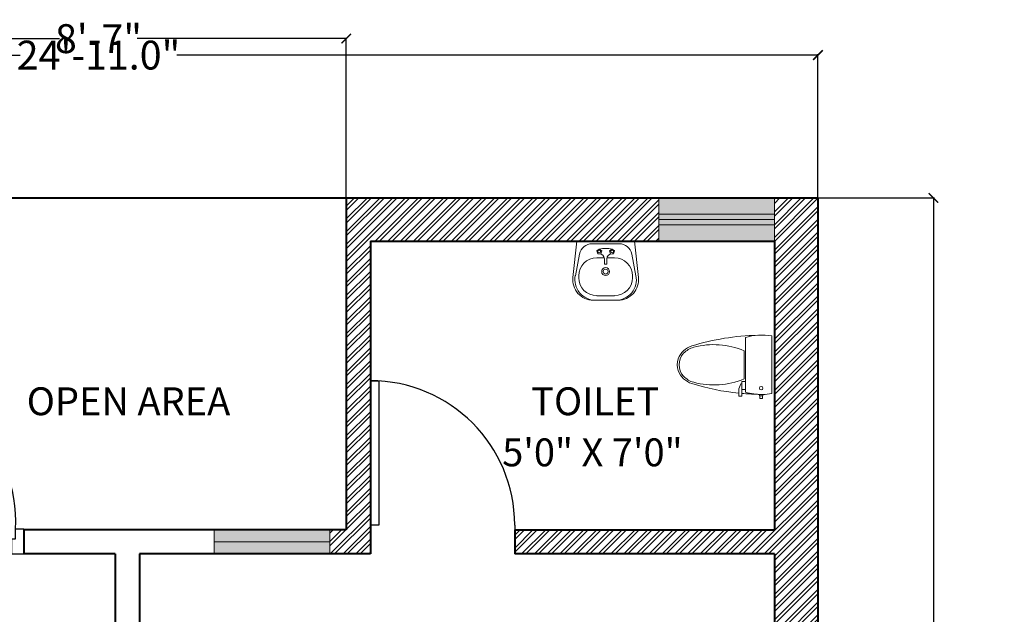
# Model space of a CAD drawing. Units: inches. Extents: x 528 to 2520, y -151 to 1354.
# Tile 14 of 41: x 720 to 924, y 1231 to 1354. Entities that reach past the tile are written whole.
import ezdxf

# ---------------------------------------------------------------- set-up
doc = ezdxf.new("R2010")
doc.units = ezdxf.units.IN
doc.header["$MEASUREMENT"] = 0
for name, color, linetype, lineweight in [('A-ANNO-DIMS', 2, 'Continuous', 18), ('A-AREA-IDEN', 7, 'Continuous', 18), ('A-Door', 150, 'Continuous', 25), ('A-FLOR-FIXT', 9, 'Continuous', 18), ('A-WALL-PATT', 6, 'Continuous', 13), ('walls', 7, 'Continuous', 40), ('WINDOWS', 2, 'Continuous', 20)]:
    doc.layers.add(name, color=color, linetype=linetype, lineweight=lineweight)
doc.layers.add('A-GLAZ-PATT', color=152, linetype='Continuous', lineweight=13, true_color=0x2776bb)
doc.layers.add('NT', color=1, linetype='Continuous')
doc.styles.get("Standard").update_dxf_attribs({"font": 'arial.ttf'})
doc.dimstyles.get("Standard").update_dxf_attribs({"dimtxt": 6, "dimasz": 2, "dimexe": 0.18, "dimexo": 0.0625, "dimgap": 0.09, "dimtad": 0, "dimtih": 1, "dimtoh": 1, "dimdec": 1, "dimzin": 0, "dimdsep": 46, "dimlunit": 3, "dimtxsty": 'Standard', "dimblk": 'ARCHTICK', "dimcen": 0.09, "dimadec": 0, "dimazin": 0, "dimtfac": 1, "dimtdec": 1, "dimtofl": 0, "dimtmove": 0, "dimatfit": 3, "dimfxl": 1, "dimtolj": 1, "dimtzin": 0, "dimarcsym": 0})

# ---------------------------------------------------------------- blocks, each defined once
blk = doc.blocks.new('A$C7DB75F4D')
at = {"layer": 'A-Door'}
for points in [[(625, 740), (625, 660), (665, 660), (665, 740)], [(625, 180), (625, 660), (665, 660), (665, 180)], [(625, 100), (625, 180), (665, 180), (665, 100)], [(35, 100), (35, 60), (50, 60), (50, 50), (50, 0), (0, 0), (0, 100)], [(665, 100), (700, 100), (700, 0), (650, 0), (650, 50), (650, 60), (665, 60)]]:
    blk.add_lwpolyline(points, close=True, dxfattribs=at)
at = {"layer": 'NT'}
blk.add_arc((650, 125), 615.5, 92.3278, 182.3278, dxfattribs=at)
blk = doc.blocks.new('toilet-7')
at = {"color": 0, "linetype": 'ByBlock'}
for p, q in [((0.2097, -0.02), (-0.2097, -0.02)), ((0.2151, -0.0677), (0.2097, -0.02)), ((0.2151, -0.1171), (0.2151, -0.0677)), ((-0.2457, -0.0874), (-0.2457, -0.1068)), ((-0.2457, -0.0874), (-0.2257, -0.0874)), ((-0.2457, -0.1068), (-0.2257, -0.1068)), ((-0.2257, -0.0846), (-0.2257, -0.1096)), ((-0.2257, -0.0846), (-0.2157, -0.0846)), ((-0.2257, -0.1096), (-0.2154, -0.1096)), ((0.2099, -0.164), (0.2151, -0.1171)), ((0.1991, -0.2124), (-0.1991, -0.2124)), ((-0.1803, -0.2374), (-0.1803, -0.2124)), ((-0.1213, -0.2374), (-0.1213, -0.2124)), ((0.1991, -0.2124), (0.2099, -0.164)), ((-0.1213, -0.2374), (-0.2278, -0.2374)), ((-0.2278, -0.2374), (-0.2278, -0.2599)), ((-0.1759, -0.2599), (-0.2278, -0.2599)), ((-0.1759, -0.2599), (-0.1379, -0.2451)), ((-0.1379, -0.2451), (-0.1379, -0.2374)), ((-0.1023, -0.2212), (0.1023, -0.2212))]:
    blk.add_line(p, q, dxfattribs=at)
blk.add_circle((-0.1696, -0.0971), 0.0125, dxfattribs=at)
for centre, radius, start, end in [((0.2244, -0.0924), 0.4402, 170.53768, 187.73995), ((1.517, -0.087), 1.7318, 181.22237, 184.98223), ((-1.517, -0.087), 1.7318, 342.75226, 358.77763), ((0.2244, -0.0924), 0.4402, 187.73995, 195.82198), ((1.517, -0.087), 1.7318, 185.73228, 197.24774), ((0.4258, -0.4413), 0.5721, 157.37374, 194.77857), ((-0.4258, -0.4413), 0.5721, 345.22143, 22.62626), ((0.0116, -0.5544), 0.1554, 197.24774, 249.54761), ((0.0221, -0.5478), 0.1546, 194.77857, 226.85426), ((-0.0116, -0.5544), 0.1554, 290.45239, 342.75226), ((-0.0221, -0.5478), 0.1546, 313.14574, 345.22143), ((0, -0.5713), 0.1223, 226.85426, 313.14574), ((0, -0.5854), 0.1223, 249.54761, 290.45239)]:
    blk.add_arc(centre, radius, start, end, dxfattribs=at)
blk = doc.blocks.new('_ArchTick')
at = {"color": 0, "linetype": 'ByBlock', "const_width": 0.15}
blk.add_lwpolyline([(-0.5, -0.5), (0.5, 0.5)], dxfattribs=at)
blk = doc.blocks.new('*D24')
at = {"layer": 'A-ANNO-DIMS', "color": 0, "lineweight": -2, "transparency": 16777216}
for p, q in [((885.76, 1317.1), (909.9, 1317.1)), ((909.72, 1317.1), (909.72, 1069.76)), ((909.72, 816.1), (909.72, 1063.45)), ((885.76, 816.1), (909.9, 816.1))]:
    blk.add_line(p, q, dxfattribs=at)
at = {"layer": 'Defpoints', "color": 0, "transparency": 16777216}
for p in [(885.7, 1317.1), (885.7, 816.1), (909.72, 816.1)]:
    blk.add_point(p, dxfattribs=at)
at = {"layer": 'A-ANNO-DIMS', "color": 0, "lineweight": -2, "transparency": 16777216, "xscale": 2, "yscale": 2, "zscale": 2}
for p, rotation in [((909.72, 1317.1), 90), ((909.72, 816.1), 270)]:
    blk.add_blockref('_ArchTick', p, dxfattribs=dict(at, rotation=rotation))
at = {"layer": 'A-ANNO-DIMS', "color": 0, "transparency": 16777216, "insert": (909.72, 1066.6), "char_height": 6, "attachment_point": 5}
blk.add_mtext('\\A1;41\'-9.0"', dxfattribs=at)
blk = doc.blocks.new('*D25')
at = {"layer": 'A-ANNO-DIMS', "color": 0, "lineweight": -2, "transparency": 16777216}
for p, q in [((586.7, 1317.17), (586.7, 1346.96)), ((586.7, 1346.78), (719.92, 1346.78)), ((885.7, 1346.78), (752.47, 1346.78)), ((885.7, 1317.17), (885.7, 1346.96))]:
    blk.add_line(p, q, dxfattribs=at)
at = {"layer": 'Defpoints', "color": 0, "transparency": 16777216}
for p in [(885.7, 1346.78), (586.7, 1317.1), (885.7, 1317.1)]:
    blk.add_point(p, dxfattribs=at)
at = {"layer": 'A-ANNO-DIMS', "color": 0, "lineweight": -2, "transparency": 16777216, "xscale": 2, "yscale": 2, "zscale": 2, "rotation": 180}
blk.add_blockref('_ArchTick', (586.7, 1346.78), dxfattribs=at)
at = {"layer": 'A-ANNO-DIMS', "color": 0, "lineweight": -2, "transparency": 16777216, "xscale": 2, "yscale": 2, "zscale": 2}
blk.add_blockref('_ArchTick', (885.7, 1346.78), dxfattribs=at)
at = {"layer": 'A-ANNO-DIMS', "color": 0, "transparency": 16777216, "insert": (736.2, 1346.78), "char_height": 6, "attachment_point": 5}
blk.add_mtext('\\A1;24\'-11.0"', dxfattribs=at)
blk = doc.blocks.new('BASIN-WITH-TAP')
for p, q in [((0.84, 12.27), (0.02, 4.73)), ((12.84, 12.27), (0.84, 12.27)), ((9.64, 11.73), (4.05, 11.73)), ((5, 10.24), (5.51, 10.61)), ((5.2, 9.64), (5, 10.24)), ((5.51, 10.61), (6.02, 10.24)), ((6.02, 10.24), (5.82, 9.64)), ((8.18, 10.61), (7.67, 10.24)), ((7.67, 10.24), (7.86, 9.64)), ((8.68, 10.24), (8.18, 10.61)), ((8.49, 9.64), (8.68, 10.24)), ((12.84, 12.27), (13.66, 4.73)), ((1.43, 9.58), (0.55, 5.09)), ((4.98, 8.8), (6.58, 8.8)), ((5.24, 10.1), (5.2, 10.1)), ((5.24, 9.64), (5.51, 9.64)), ((6.58, 8.31), (6.58, 8.58)), ((6.58, 7.51), (6.58, 8.31)), ((8.71, 8.8), (7.11, 8.8)), ((7.11, 8.31), (7.11, 8.58)), ((7.11, 7.51), (7.11, 8.31)), ((8.49, 9.64), (8.18, 9.64)), ((8.44, 10.1), (8.49, 10.1)), ((12.26, 9.58), (13.14, 5.09)), ((6.58, 7.51), (7.11, 7.51)), ((1.24, 4.67), (1.24, 5.07)), ((12.44, 4.67), (12.44, 5.07)), ((4.73, 0), (8.96, 0)), ((6.84, 0.93), (4.98, 0.93)), ((6.84, 0.93), (8.71, 0.93))]:
    blk.add_line(p, q)
for centre, radius in [((5.5, 10.1), 0.277), ((8.19, 10.1), 0.277), ((6.84, 5.94), 0.821), ((6.84, 5.94), 0.507)]:
    blk.add_circle(centre, radius)
for centre, radius, start, end in [((4.05, 9.07), 2.67, 90, 168.8773), ((6.84, 4.01), 6.73, 78.5788, 101.4212), ((9.64, 9.07), 2.67, 11.1227, 90), ((4.98, 5.07), 3.73, 90, 180), ((5.51, 8.58), 1.07, 0, 90), ((8.18, 8.58), 1.07, 90, 180), ((8.71, 5.07), 3.73, 0, 90), ((4.27, 4.27), 4.27, 173.7966, 270), ((4.73, 4.27), 4.27, 168.8773, 270), ((4.98, 4.67), 3.73, 180, 270), ((8.71, 4.67), 3.73, 270, 0), ((8.96, 4.27), 4.27, 270, 11.1227), ((9.42, 4.27), 4.27, 270, 6.2034)]:
    blk.add_arc(centre, radius, start, end)
blk = doc.blocks.new('DOOR-SWING-30')
for p, q in [((0, 6), (0, 0)), ((30, 6), (30, 0))]:
    blk.add_line(p, q)
blk.add_lwpolyline([(0, 6), (0, 36), (1.75, 36), (1.75, 6)], close=True)
blk.add_arc((0, 6), 30, 0, 90)
blk = doc.blocks.new('WINDOW-24x9-PLAN')
for p, q in [((0, 5.63), (24, 5.63)), ((0, 4.5), (24, 4.5)), ((0, 3.37), (24, 3.37))]:
    blk.add_line(p, q)
blk.add_lwpolyline([(0, 9), (24, 9), (24, 0), (0, 0)], close=True)
blk = doc.blocks.new('WINDOW-24x5-PLAN')
for p, q in [((0, 5), (24, 5)), ((24, 0), (24, 5)), ((0, 2.5), (24, 2.5))]:
    blk.add_line(p, q)
blk.add_lwpolyline([(0, 5), (24, 5), (24, 0), (0, 0)], close=True)
blk = doc.blocks.new('*D93')
at = {"layer": 'A-ANNO-DIMS', "color": 0, "lineweight": -2, "transparency": 16777216}
for p, q in [((684.7, 1317.17), (684.7, 1350.38)), ((684.7, 1350.2), (728.13, 1350.2)), ((787.7, 1350.2), (744.27, 1350.2)), ((787.7, 1317.17), (787.7, 1350.38))]:
    blk.add_line(p, q, dxfattribs=at)
at = {"layer": 'Defpoints', "color": 0, "transparency": 16777216}
for p in [(787.7, 1350.2), (684.7, 1317.1), (787.7, 1317.1)]:
    blk.add_point(p, dxfattribs=at)
at = {"layer": 'A-ANNO-DIMS', "color": 0, "lineweight": -2, "transparency": 16777216, "xscale": 2, "yscale": 2, "zscale": 2, "rotation": 180}
blk.add_blockref('_ArchTick', (684.7, 1350.2), dxfattribs=at)
at = {"layer": 'A-ANNO-DIMS', "color": 0, "lineweight": -2, "transparency": 16777216, "xscale": 2, "yscale": 2, "zscale": 2}
blk.add_blockref('_ArchTick', (787.7, 1350.2), dxfattribs=at)
at = {"layer": 'A-ANNO-DIMS', "color": 0, "transparency": 16777216, "insert": (736.2, 1350.2), "char_height": 6, "attachment_point": 5}
blk.add_mtext('\\A1;8\'-7"', dxfattribs=at)

msp = doc.modelspace()

# ---------------------------------------------------------------- hatches: boundary and pattern name
at = {"layer": 'A-GLAZ-PATT'}
h = msp.add_hatch(color=256, dxfattribs=at)
h.dxf.hatch_style = 1
h.paths.add_polyline_path([(876.65, 1313.73), (852.65, 1313.73), (852.65, 1312.6), (876.65, 1312.6)])
h.paths.add_polyline_path([(876.65, 1312.6), (852.65, 1312.6), (852.65, 1311.47), (876.65, 1311.47)])
h.paths.add_polyline_path([(876.65, 1317.1), (852.65, 1317.1), (852.65, 1313.73), (876.65, 1313.73)])
h.paths.add_polyline_path([(876.65, 1311.47), (852.65, 1311.47), (852.65, 1308.1), (876.65, 1308.1)])
h = msp.add_hatch(color=256, dxfattribs=at)
h.dxf.hatch_style = 1
h.paths.add_polyline_path([(784.26, 1248.1), (760.26, 1248.1), (760.26, 1245.6), (784.26, 1245.6)])
h.paths.add_polyline_path([(784.26, 1245.6), (760.26, 1245.6), (760.26, 1243.1), (784.26, 1243.1)])
at = {"layer": 'A-WALL-PATT'}
h = msp.add_hatch(dxfattribs=at)
h.set_pattern_fill('ANSI32', color=256, scale=5)
h.paths.add_polyline_path([(595.7, 1163.86), (586.7, 1163.86), (586.7, 969.1), (598.24, 969.1), (603.24, 969.1), (603.24, 974.1), (595.7, 974.1), (595.7, 1082.1), (691.7, 1082.1), (691.7, 1087.1), (691.7, 1106.1), (697.7, 1106.1), (697.7, 1111.1), (686.7, 1111.1), (686.7, 1087.1), (595.7, 1087.1)])
h.paths.add_polyline_path([(688.7, 974.1), (651.24, 974.1), (651.24, 969.1), (688.7, 969.1)])
h.paths.add_polyline_path([(885.7, 1171.37), (876.7, 1171.37), (876.7, 1111.1), (786.7, 1111.1), (786.7, 1106.1), (876.7, 1106.1), (876.7, 974.1), (786.7, 974.1), (786.7, 969.1), (876.7, 969.1), (876.7, 825.1), (834.7, 825.1), (834.7, 816.1), (885.7, 816.1)])
h.paths.add_polyline_path([(885.7, 1317.1), (876.65, 1317.1), (876.65, 1308.1), (876.7, 1308.1), (876.7, 1248.1), (822.7, 1248.1), (822.7, 1243.1), (876.7, 1243.1), (876.7, 1219.37), (885.7, 1219.37)])
h.paths.add_polyline_path([(852.65, 1317.1), (787.7, 1317.1), (787.7, 1248.1), (784.26, 1248.1), (784.26, 1243.1), (792.7, 1243.1), (792.7, 1249.1), (792.7, 1308.1), (852.65, 1308.1)])
h.paths.add_polyline_path([(684.7, 1317.1), (619.7, 1317.1), (619.7, 1308.1), (679.7, 1308.1), (679.7, 1248.1), (679.7, 1243.1), (684.7, 1243.1), (684.7, 1248.25)])
h.paths.add_polyline_path([(595.7, 1308.1), (595.7, 1317.1), (586.7, 1317.1), (586.7, 1211.86), (595.7, 1211.86), (595.7, 1243.1), (649.7, 1243.1), (649.7, 1248.1), (595.7, 1248.1)])
h.paths.add_polyline_path([(744.7, 969.1), (744.7, 974.1), (724.7, 974.1), (724.7, 969.1), (739.7, 969.1), (739.7, 874.29), (744.7, 874.29)])
h.paths.add_polyline_path([(739.7, 969.1), (727.7, 969.1), (727.7, 965.12), (730.74, 965.12), (730.74, 961.68), (734.43, 961.68), (734.43, 957.24), (739.7, 957.24)], flags=17)
h.paths.add_polyline_path([(786.7, 825.1), (744.7, 825.1), (744.7, 832.29), (739.7, 832.29), (739.7, 816.1), (786.7, 816.1)])

# ---------------------------------------------------------------- linework, layer by layer
at = {"layer": 'walls'}
for p, q in [((684.7, 1317.1), (787.7, 1317.1)), ((787.7, 1317.1), (885.7, 1317.1)), ((787.7, 1317.1), (787.7, 1248.1)), ((885.7, 1317.1), (885.7, 816.1)), ((792.7, 1308.1), (876.7, 1308.1)), ((792.7, 1308.1), (792.7, 1248.1)), ((876.7, 1308.1), (876.7, 1248.1)), ((787.7, 1248.1), (720.7, 1248.1)), ((720.7, 1248.1), (720.7, 1243.1)), ((792.7, 1248.1), (792.7, 1243.1)), ((822.7, 1248.1), (876.7, 1248.1)), ((822.7, 1248.1), (822.7, 1243.1)), ((739.7, 1243.1), (720.7, 1243.1)), ((739.7, 1243.1), (739.7, 1111.1)), ((744.7, 1243.1), (744.7, 1111.1)), ((792.7, 1243.1), (744.7, 1243.1)), ((876.7, 1243.1), (822.7, 1243.1)), ((876.7, 1243.1), (876.7, 1111.1))]:
    msp.add_line(p, q, dxfattribs=at)

# ---------------------------------------------------------------- block references
at = {"layer": 'A-Door', "xscale": -0.0514539602427209, "yscale": 0.0514539602427209, "zscale": 0.0514539602427209}
msp.add_blockref('A$C7DB75F4D', (720.71, 1243.1), dxfattribs=at)
at = {"layer": 'A-Door'}
msp.add_blockref('DOOR-SWING-30', (792.7, 1243.1), dxfattribs=at)
at = {"layer": 'A-FLOR-FIXT'}
msp.add_blockref('BASIN-WITH-TAP', (834.75, 1295.84), dxfattribs=at)
at = {"layer": 'A-FLOR-FIXT', "xscale": -28.60654769571749, "yscale": 28.60654769571749, "zscale": 28.60654769571749, "rotation": 270}
msp.add_blockref('toilet-7', (876.7, 1282.41), dxfattribs=at)
at = {"layer": 'WINDOWS'}
for name, p in [('WINDOW-24x9-PLAN', (852.65, 1308.1)), ('WINDOW-24x5-PLAN', (760.26, 1243.1))]:
    msp.add_blockref(name, p, dxfattribs=at)

# ---------------------------------------------------------------- texts
at = {"layer": 'A-AREA-IDEN'}
for s, height, p in [('OPEN AREA', 5.793, (721.29, 1271.93)), ('TOILET', 5.793, (826.12, 1271.93)), ('5\'0" X 7\'0"', 5.7926, (820.1, 1261.31))]:
    msp.add_text(s, height=height, dxfattribs=at).set_placement(p)

# ---------------------------------------------------------------- dimensions: what is measured, and where the dimension line sits
at = {"layer": 'A-ANNO-DIMS'}
for base, p1, p2, override, picture, middle in [((787.7, 1350.2), (684.7, 1317.1), (787.7, 1317.1), {"dimdec": 1, "dimlfac": 1, "dimrnd": 0, "dimzin": 1, "dimdsep": 46, "dimlunit": 4, "dimfrac": 2}, '*D93', (736.2, 1350.2)), ((885.7, 1346.78), (586.7, 1317.1), (885.7, 1317.1), {"dimclrd": 0, "dimclre": 0, "dimclrt": 0}, '*D25', (736.2, 1346.78))]:
    dim = msp.add_linear_dim(base=base, p1=p1, p2=p2, dimstyle='Standard', override=override, dxfattribs=at)
    dim.commit()
    dim.dimension.update_dxf_attribs({"geometry": picture, "text_midpoint": middle})
dim = msp.add_linear_dim(base=(909.72, 816.1), p1=(885.7, 1317.1), p2=(885.7, 816.1), angle=90, dimstyle='Standard', override={"dimclrd": 0, "dimclre": 0, "dimclrt": 0}, dxfattribs=at)
dim.commit()
dim.dimension.update_dxf_attribs({"geometry": '*D24', "text_midpoint": (909.72, 1066.6)})

doc.saveas('drawing.dxf')
